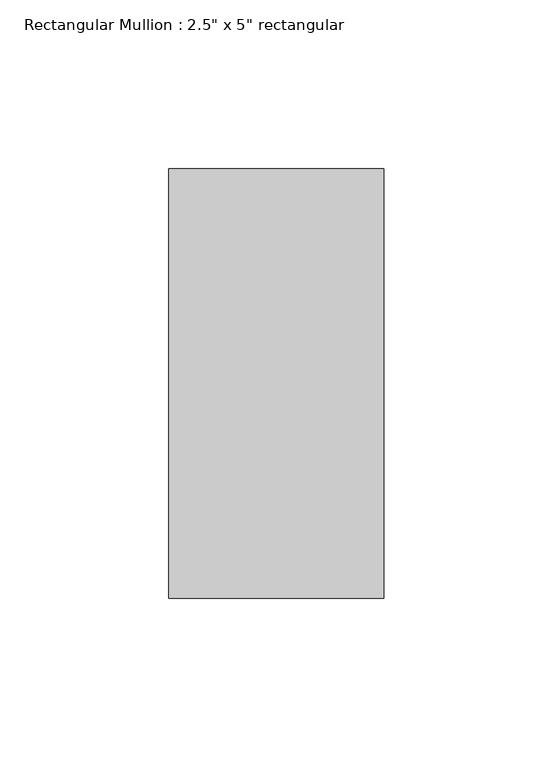
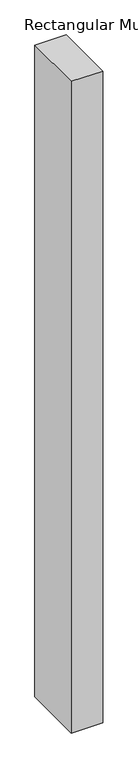
"""IFC4 building model written with IfcOpenShell, lengths in millimetres: member geometry."""

from ifc_helpers import new_model, si_unit, frame, origin, place, context, project, spatial, polyline, outline, extrude, source, transform, mapped, element, save


def member_1929af86(model_context):
    return source(origin(), model_context, "Body", "SweptSolid", [
        extrude(outline(polyline([(0.0, 63.5), (0.0, -63.5), (-63.5, -63.5), (-63.5, 63.5), (0.0, 63.5)])), frame((0.0, 0.0, -1388.8321364), z_axis=(0.0, 0.0, 1.0), x_axis=(1.0, 0.0, 0.0)), (0.0, 0.0, 1.0), 1388.8321364),
    ])


if __name__ == "__main__":
    model = new_model("IFC4")
    model_context = context("Model", 3, world=origin())
    ifc_project = project(units=[si_unit("LENGTHUNIT", "METRE", prefix="MILLI")], contexts=[model_context])
    site = spatial("IfcSite", under=ifc_project)
    building = spatial("IfcBuilding", under=site)
    placement = place(None, origin())
    member_shape = member_1929af86(model_context)
    element("IfcMember", 1, ObjectType="Rectangular Mullion : 2.5\" x 5\" rectangular", at=placement, inside=building, context=model_context, shape_type="MappedRepresentation", body=[
        mapped(member_shape, transform((0.0, 0.0, 0.0), x_axis=(1.0, 0.0, 0.0), y_axis=(0.0, 1.0, 0.0), z_axis=(0.0, 0.0, 1.0))),
    ])
    save(model, "model.ifc")

# Revit data of these elements
# Type "Rectangular Mullion : 2.5\" x 5\" rectangular"
#   built-in parameter 1007304 = 0.416667 (stored number, unit not read)
#   built-in parameter 1007301 = 0.104167 (stored number, unit not read)
#   built-in parameter 1007300 = 0.104167 (stored number, unit not read)
# Element 1 (IfcMember, "Rectangular Mullion : 2.5\" x 5\" rectangular")
#   Materials on its faces: "Aluminum"
# Materials
#   "Aluminum": class "Metal", colour RGB 247 247 247, transparency 0, Description = "Aluminum 6061", Cost = 0
